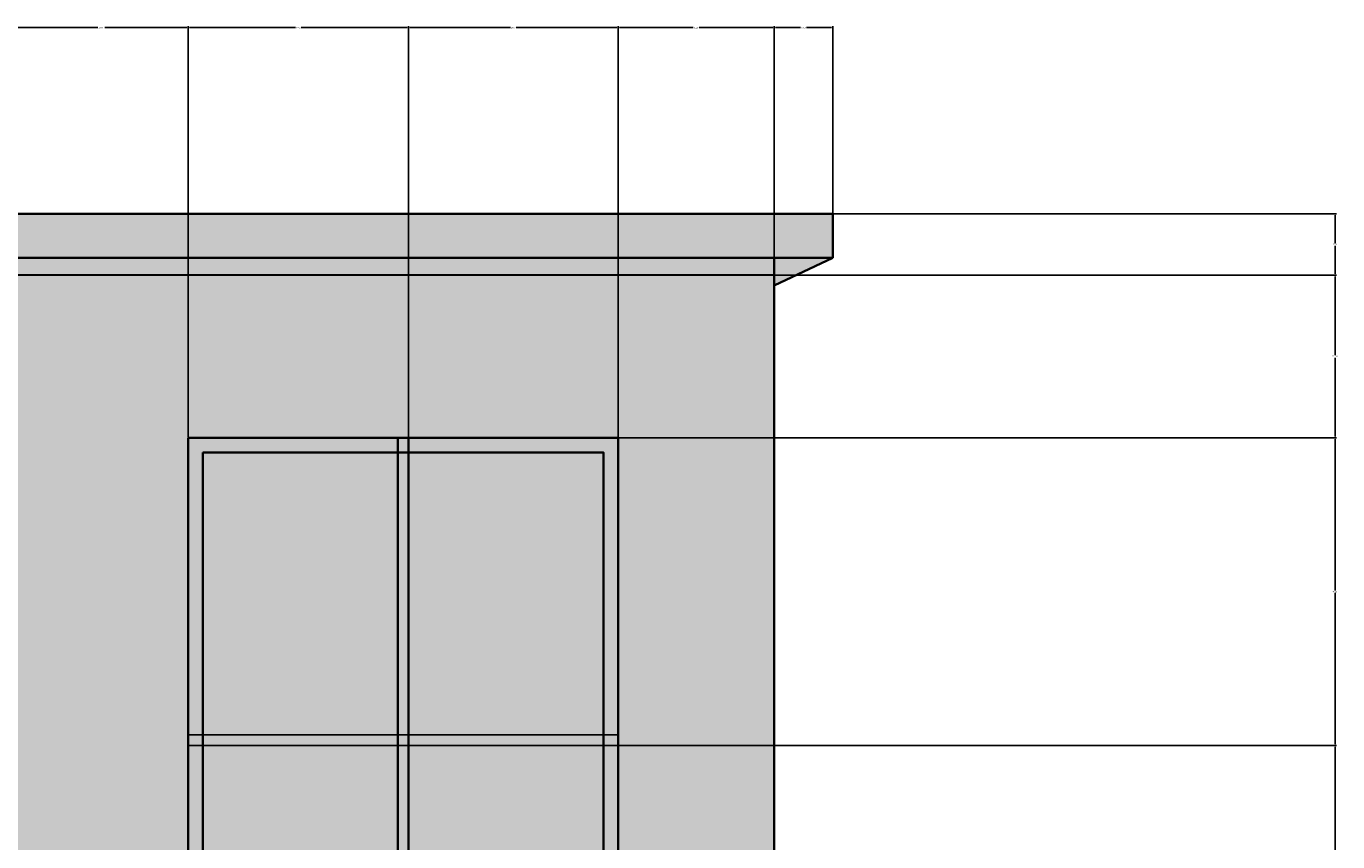
# Model space of a CAD drawing. Units: feet. Extents: x 2415 to 6174, y 866 to 1295.
# Tile 6 of 9: x 3580 to 3759, y 1184 to 1295. Entities that reach past the tile are written whole.
import ezdxf

# ---------------------------------------------------------------- set-up
doc = ezdxf.new("R2010")
doc.units = ezdxf.units.FT
for name, color, linetype, lineweight in [('A-ANNO-DIMS', 2, 'Continuous', 18), ('A-ELEV', 7, 'Continuous', 35), ('A-ELEV-PATT', 8, 'Continuous', 13), ('A-GLAZ', 4, 'Continuous', 25)]:
    doc.layers.add(name, color=color, linetype=linetype, lineweight=lineweight)
doc.styles.get("Standard").update_dxf_attribs({"font": 'arial.ttf'})
doc.dimstyles.get("Standard").update_dxf_attribs({"dimtxt": 0.18, "dimasz": 0.18, "dimexe": 0.18, "dimexo": 0.0625, "dimgap": 0.09, "dimtad": 0, "dimtih": 1, "dimtoh": 1, "dimdec": 1, "dimzin": 0, "dimdsep": 46, "dimlunit": 3, "dimtxsty": 'Standard', "dimcen": 0.09, "dimadec": 0, "dimazin": 0, "dimtfac": 1, "dimtdec": 1, "dimtofl": 0, "dimtmove": 0, "dimatfit": 3, "dimfxl": 1, "dimtolj": 1, "dimtzin": 0, "dimarcsym": 0})

# ---------------------------------------------------------------- blocks, each defined once
blk = doc.blocks.new('*D67')
at = {"layer": 'A-ANNO-DIMS', "color": 0, "lineweight": -2, "transparency": 16777216}
for p, q in [((3578.56, 1263.66), (3578.56, 1295.18)), ((3578.74, 1295), (3589.92, 1295)), ((3602.04, 1295), (3590.85, 1295)), ((3602.22, 1239.13), (3602.22, 1295.18))]:
    blk.add_line(p, q, dxfattribs=at)
at = {"layer": 'A-ANNO-DIMS', "color": 0, "transparency": 16777216}
for points in [[(3578.74, 1295.03), (3578.74, 1294.97), (3578.56, 1295)], [(3602.04, 1295.03), (3602.04, 1294.97), (3602.22, 1295)]]:
    blk.add_solid(points, dxfattribs=at)
at = {"layer": 'Defpoints', "color": 0, "transparency": 16777216}
for p in [(3602.22, 1295), (3578.56, 1263.6), (3602.22, 1239.07)]:
    blk.add_point(p, dxfattribs=at)
at = {"layer": 'A-ANNO-DIMS', "color": 0, "transparency": 16777216, "insert": (3590.39, 1295), "char_height": 0.18, "attachment_point": 5}
blk.add_mtext('\\A1;23.657', dxfattribs=at)
blk = doc.blocks.new('*D68')
at = {"layer": 'A-ANNO-DIMS', "color": 0, "lineweight": -2, "transparency": 16777216}
for p, q in [((3602.22, 1239.13), (3602.22, 1295.18)), ((3602.4, 1295), (3616.84, 1295)), ((3632.06, 1295), (3617.62, 1295)), ((3632.24, 1239.13), (3632.24, 1295.18))]:
    blk.add_line(p, q, dxfattribs=at)
at = {"layer": 'A-ANNO-DIMS', "color": 0, "transparency": 16777216}
for points in [[(3602.4, 1295.03), (3602.4, 1294.97), (3602.22, 1295)], [(3632.06, 1295.03), (3632.06, 1294.97), (3632.24, 1295)]]:
    blk.add_solid(points, dxfattribs=at)
at = {"layer": 'Defpoints', "color": 0, "transparency": 16777216}
for p in [(3632.24, 1295), (3602.22, 1239.07), (3632.24, 1239.07)]:
    blk.add_point(p, dxfattribs=at)
at = {"layer": 'A-ANNO-DIMS', "color": 0, "transparency": 16777216, "insert": (3617.23, 1295), "char_height": 0.18, "attachment_point": 5}
blk.add_mtext('\\A1;30.03', dxfattribs=at)
blk = doc.blocks.new('*D69')
at = {"layer": 'A-ANNO-DIMS', "color": 0, "lineweight": -2, "transparency": 16777216}
for p, q in [((3632.24, 1239.13), (3632.24, 1295.18)), ((3632.42, 1295), (3646.13, 1295)), ((3660.63, 1295), (3646.92, 1295)), ((3660.81, 1239.13), (3660.81, 1295.18))]:
    blk.add_line(p, q, dxfattribs=at)
at = {"layer": 'A-ANNO-DIMS', "color": 0, "transparency": 16777216}
for points in [[(3632.42, 1295.03), (3632.42, 1294.97), (3632.24, 1295)], [(3660.63, 1295.03), (3660.63, 1294.97), (3660.81, 1295)]]:
    blk.add_solid(points, dxfattribs=at)
at = {"layer": 'Defpoints', "color": 0, "transparency": 16777216}
for p in [(3660.81, 1295), (3632.24, 1239.07), (3660.81, 1239.07)]:
    blk.add_point(p, dxfattribs=at)
at = {"layer": 'A-ANNO-DIMS', "color": 0, "transparency": 16777216, "insert": (3646.53, 1295), "char_height": 0.18, "attachment_point": 5}
blk.add_mtext('\\A1;28.57', dxfattribs=at)
blk = doc.blocks.new('*D70')
at = {"layer": 'A-ANNO-DIMS', "color": 0, "lineweight": -2, "transparency": 16777216}
for p, q in [((3660.81, 1239.13), (3660.81, 1295.18)), ((3660.99, 1295), (3671.05, 1295)), ((3681.89, 1295), (3671.84, 1295)), ((3682.07, 1261.33), (3682.07, 1295.18))]:
    blk.add_line(p, q, dxfattribs=at)
at = {"layer": 'A-ANNO-DIMS', "color": 0, "transparency": 16777216}
for points in [[(3660.99, 1295.03), (3660.99, 1294.97), (3660.81, 1295)], [(3681.89, 1295.03), (3681.89, 1294.97), (3682.07, 1295)]]:
    blk.add_solid(points, dxfattribs=at)
at = {"layer": 'Defpoints', "color": 0, "transparency": 16777216}
for p in [(3682.07, 1295), (3682.07, 1261.26), (3660.81, 1239.07)]:
    blk.add_point(p, dxfattribs=at)
at = {"layer": 'A-ANNO-DIMS', "color": 0, "transparency": 16777216, "insert": (3671.44, 1295), "char_height": 0.18, "attachment_point": 5}
blk.add_mtext('\\A1;21.26', dxfattribs=at)
blk = doc.blocks.new('*D71')
at = {"layer": 'A-ANNO-DIMS', "color": 0, "lineweight": -2, "transparency": 16777216}
for p, q in [((3682.07, 1261.33), (3682.07, 1295.18)), ((3682.25, 1295), (3685.69, 1295)), ((3689.91, 1295), (3686.48, 1295)), ((3690.09, 1269.66), (3690.09, 1295.18))]:
    blk.add_line(p, q, dxfattribs=at)
at = {"layer": 'A-ANNO-DIMS', "color": 0, "transparency": 16777216}
for points in [[(3682.25, 1295.03), (3682.25, 1294.97), (3682.07, 1295)], [(3689.91, 1295.03), (3689.91, 1294.97), (3690.09, 1295)]]:
    blk.add_solid(points, dxfattribs=at)
at = {"layer": 'Defpoints', "color": 0, "transparency": 16777216}
for p in [(3690.09, 1295), (3690.09, 1269.6), (3682.07, 1261.26)]:
    blk.add_point(p, dxfattribs=at)
at = {"layer": 'A-ANNO-DIMS', "color": 0, "transparency": 16777216, "insert": (3686.08, 1295), "char_height": 0.18, "attachment_point": 5}
blk.add_mtext('\\A1;8.019', dxfattribs=at)
blk = doc.blocks.new('*D86')
at = {"layer": 'A-ANNO-DIMS', "color": 0, "lineweight": -2, "transparency": 16777216}
for p, q in [((3660.88, 1197.11), (3758.71, 1197.11)), ((3758.53, 1196.93), (3758.53, 1177.05)), ((3758.53, 1156.8), (3758.53, 1176.69)), ((3660.88, 1156.62), (3758.71, 1156.62))]:
    blk.add_line(p, q, dxfattribs=at)
at = {"layer": 'A-ANNO-DIMS', "color": 0, "transparency": 16777216}
for points in [[(3758.5, 1196.93), (3758.56, 1196.93), (3758.53, 1197.11)], [(3758.5, 1156.8), (3758.56, 1156.8), (3758.53, 1156.62)]]:
    blk.add_solid(points, dxfattribs=at)
at = {"layer": 'Defpoints', "color": 0, "transparency": 16777216}
for p in [(3660.81, 1197.11), (3758.53, 1197.11), (3660.81, 1156.62)]:
    blk.add_point(p, dxfattribs=at)
at = {"layer": 'A-ANNO-DIMS', "color": 0, "transparency": 16777216, "insert": (3758.53, 1176.87), "char_height": 0.18, "attachment_point": 5}
blk.add_mtext('\\A1;40.49', dxfattribs=at)
blk = doc.blocks.new('*D87')
at = {"layer": 'A-ANNO-DIMS', "color": 0, "lineweight": -2, "transparency": 16777216}
for p, q in [((3660.88, 1239.07), (3758.71, 1239.07)), ((3758.53, 1238.89), (3758.53, 1218.27)), ((3758.53, 1197.29), (3758.53, 1217.91)), ((3660.88, 1197.11), (3758.71, 1197.11))]:
    blk.add_line(p, q, dxfattribs=at)
at = {"layer": 'A-ANNO-DIMS', "color": 0, "transparency": 16777216}
for points in [[(3758.5, 1238.89), (3758.56, 1238.89), (3758.53, 1239.07)], [(3758.5, 1197.29), (3758.56, 1197.29), (3758.53, 1197.11)]]:
    blk.add_solid(points, dxfattribs=at)
at = {"layer": 'Defpoints', "color": 0, "transparency": 16777216}
for p in [(3660.81, 1239.07), (3758.53, 1239.07), (3660.81, 1197.11)]:
    blk.add_point(p, dxfattribs=at)
at = {"layer": 'A-ANNO-DIMS', "color": 0, "transparency": 16777216, "insert": (3758.53, 1218.09), "char_height": 0.18, "attachment_point": 5}
blk.add_mtext('\\A1;41.95', dxfattribs=at)
blk = doc.blocks.new('*D88')
at = {"layer": 'A-ANNO-DIMS', "color": 0, "lineweight": -2, "transparency": 16777216}
for p, q in [((3682.13, 1261.26), (3758.71, 1261.26)), ((3758.53, 1261.08), (3758.53, 1250.35)), ((3758.53, 1239.25), (3758.53, 1249.98)), ((3660.88, 1239.07), (3758.71, 1239.07))]:
    blk.add_line(p, q, dxfattribs=at)
at = {"layer": 'A-ANNO-DIMS', "color": 0, "transparency": 16777216}
for points in [[(3758.5, 1261.08), (3758.56, 1261.08), (3758.53, 1261.26)], [(3758.5, 1239.25), (3758.56, 1239.25), (3758.53, 1239.07)]]:
    blk.add_solid(points, dxfattribs=at)
at = {"layer": 'Defpoints', "color": 0, "transparency": 16777216}
for p in [(3682.07, 1261.26), (3758.53, 1261.26), (3660.81, 1239.07)]:
    blk.add_point(p, dxfattribs=at)
at = {"layer": 'A-ANNO-DIMS', "color": 0, "transparency": 16777216, "insert": (3758.53, 1250.16), "char_height": 0.18, "attachment_point": 5}
blk.add_mtext('\\A1;22.196', dxfattribs=at)
blk = doc.blocks.new('*D89')
at = {"layer": 'A-ANNO-DIMS', "color": 0, "lineweight": -2, "transparency": 16777216}
for p, q in [((3690.15, 1269.6), (3758.71, 1269.6)), ((3758.53, 1269.42), (3758.53, 1265.61)), ((3758.53, 1261.44), (3758.53, 1265.25)), ((3682.13, 1261.26), (3758.71, 1261.26))]:
    blk.add_line(p, q, dxfattribs=at)
at = {"layer": 'A-ANNO-DIMS', "color": 0, "transparency": 16777216}
for points in [[(3758.5, 1269.42), (3758.56, 1269.42), (3758.53, 1269.6)], [(3758.5, 1261.44), (3758.56, 1261.44), (3758.53, 1261.26)]]:
    blk.add_solid(points, dxfattribs=at)
at = {"layer": 'Defpoints', "color": 0, "transparency": 16777216}
for p in [(3690.09, 1269.6), (3758.53, 1269.6), (3682.07, 1261.26)]:
    blk.add_point(p, dxfattribs=at)
at = {"layer": 'A-ANNO-DIMS', "color": 0, "transparency": 16777216, "insert": (3758.53, 1265.43), "char_height": 0.18, "attachment_point": 5}
blk.add_mtext('\\A1;8.336', dxfattribs=at)

msp = doc.modelspace()

# ---------------------------------------------------------------- hatches: boundary and pattern name
at = {"layer": 'A-ELEV-PATT'}
h = msp.add_hatch(color=256, dxfattribs=at)
h.set_gradient(color1=(255, 255, 255), tint=1)
h.paths.add_polyline_path([(3264.916, 1143.5993), (3253.129, 1143.5993), (3253.129, 891.5993), (3264.916, 891.5993)])
h.paths.add_polyline_path([(3470.0448, 1143.5993), (3264.916, 1143.5993), (3264.916, 1137.5993), (3466.5999, 1137.5993)])
h.paths.add_polyline_path([(3363.8667, 1137.5993), (3264.916, 1137.5993), (3264.916, 1011.5993), (3363.8667, 1011.5993)])
h.paths.add_polyline_path([(3286.0429, 1117.0591), (3337.7904, 1117.0591), (3337.7904, 1115.4381), (3336.5314, 1115.4381), (3336.5314, 1110.528), (3335.4882, 1110.528), (3335.4882, 1042.3194), (3288.3452, 1042.3194), (3288.3452, 1110.528), (3287.3019, 1110.528), (3287.3019, 1115.4381), (3286.0429, 1115.4381)], flags=16)
h.paths.add_polyline_path([(3290.3452, 1108.528), (3333.4882, 1108.528), (3333.4882, 1044.3194), (3290.3452, 1044.3194)], flags=0)
h.paths.add_polyline_path([(3292.3452, 1106.528), (3331.4882, 1106.528), (3331.4882, 1046.3194), (3292.3452, 1046.3194)], flags=0)
h.paths.add_polyline_path([(3311.7156, 1106.528), (3312.1178, 1106.528), (3312.1178, 1046.3194), (3311.7156, 1046.3194)], flags=0)
h.paths.add_polyline_path([(3682.0722, 1263.5992), (3578.5579, 1263.5992), (3578.5579, 1137.5993), (3578.5579, 961.3655), (3682.0722, 961.3655)])
h.paths.add_polyline_path([(3660.8129, 1239.0671), (3660.8129, 996.6447), (3602.2151, 996.6447), (3602.2151, 1239.0671)], flags=16)
h.paths.add_polyline_path([(3632.2447, 1239.0671), (3632.2447, 996.6447), (3630.7833, 996.6447), (3630.7833, 1029.3019), (3602.2151, 1029.3019), (3602.2151, 1030.7632), (3630.7833, 1030.7632), (3630.7833, 1071.2549), (3602.2151, 1071.2549), (3602.2151, 1072.7163), (3630.7833, 1072.7163), (3630.7833, 1113.2079), (3602.2151, 1113.2079), (3602.2151, 1114.6693), (3630.7833, 1114.6693), (3630.7833, 1155.161), (3602.2151, 1155.161), (3602.2151, 1156.6224), (3630.7833, 1156.6224), (3630.7833, 1197.114), (3602.2151, 1197.114), (3602.2151, 1198.5754), (3630.7833, 1198.5754), (3630.7833, 1239.0671)], flags=0)
h.paths.add_polyline_path([(3733.129, 951.5993), (3634.5374, 951.5993), (3634.5374, 891.5993), (3733.129, 891.5993)])
h.paths.add_polyline_path([(3627.8799, 951.5993), (3621.0953, 951.5993), (3621.0953, 891.5993), (3627.8799, 891.5993)])
h.paths.add_polyline_path([(3614.4378, 951.5993), (3607.6532, 951.5993), (3607.6532, 891.5993), (3614.4378, 891.5993)])
h.paths.add_polyline_path([(3565.9347, 951.5993), (3441.3079, 951.5993), (3441.3079, 891.5993), (3565.9347, 891.5993)], flags=17)
h.paths.add_polyline_path([(3571.9347, 957.5993), (3435.3079, 957.5993), (3435.3079, 891.5993), (3441.3079, 891.5993), (3441.3079, 951.5993), (3565.9347, 951.5993), (3565.9347, 891.5993), (3571.9347, 891.5993)])
h.paths.add_polyline_path([(3435.3079, 1011.5993), (3423.5209, 1011.5993), (3423.5209, 891.5993), (3435.3079, 891.5993), (3435.3079, 957.5993)])
h.paths.add_polyline_path([(3690.0912, 1269.5992), (3571.9347, 1269.5992), (3571.9347, 1263.5992), (3690.0912, 1263.5992)])
h.paths.add_polyline_path([(3571.9347, 1269.5992), (3538.5122, 1257.6449), (3538.5122, 1251.6449), (3571.9347, 1263.5992)])
h = msp.add_hatch(color=256, dxfattribs=at)
h.set_gradient(color1=(205, 105, 40), color2=(205, 105, 40))
h.paths.add_polyline_path([(3682.0722, 1263.5992), (3578.5579, 1263.5992), (3578.5579, 1261.2323), (3682.0722, 1261.2628)])
h.paths.add_polyline_path([(3571.9347, 1261.2303), (3571.9347, 1263.5992), (3538.5122, 1251.6449), (3538.5466, 1251.5295), (3544.7493, 1251.5295), (3545.1353, 1251.6449)])
h.paths.add_polyline_path([(3578.5579, 1263.5992), (3571.9347, 1263.5992), (3571.9347, 1261.2303)])
h.paths.add_polyline_path([(3690.0912, 1263.5992), (3682.0722, 1263.5992), (3682.0722, 1261.2628), (3682.0722, 1259.8122)])
h = msp.add_hatch(color=256, dxfattribs=at)
h.set_gradient(color1=(99, 100, 102), color2=(99, 100, 102))
h.paths.add_polyline_path([(3660.8129, 1239.0671), (3602.2151, 1239.0671), (3602.2151, 996.6447), (3660.8129, 996.6447)])
h.paths.add_polyline_path([(3604.2151, 1237.0671), (3658.8129, 1237.0671), (3658.8129, 998.6447), (3604.2151, 998.6447)], flags=16)
h = msp.add_hatch(color=256, dxfattribs=at)
h.set_gradient(color1=(181, 210, 237), color2=(122, 175, 223))
h.paths.add_polyline_path([(3630.7833, 1239.0671), (3602.2151, 1239.0671), (3602.2151, 1198.5754), (3630.7833, 1198.5754)])
h.paths.add_polyline_path([(3660.8129, 1239.0671), (3632.2447, 1239.0671), (3632.2447, 1198.5754), (3660.8129, 1198.5754)])
h.paths.add_polyline_path([(3630.7833, 1197.114), (3602.2151, 1197.114), (3602.2151, 1156.6224), (3630.7833, 1156.6224)])
h.paths.add_polyline_path([(3660.8129, 1197.114), (3632.2447, 1197.114), (3632.2447, 1156.6224), (3660.8129, 1156.6224)])
h.paths.add_polyline_path([(3630.7833, 1155.161), (3602.2151, 1155.161), (3602.2151, 1114.6693), (3630.7833, 1114.6693)])
h.paths.add_polyline_path([(3660.8129, 1155.161), (3632.2447, 1155.161), (3632.2447, 1114.6693), (3660.8129, 1114.6693)])
h.paths.add_polyline_path([(3630.7833, 1113.2079), (3602.2151, 1113.2079), (3602.2151, 1072.7163), (3630.7833, 1072.7163)])
h.paths.add_polyline_path([(3660.8129, 1113.2079), (3632.2447, 1113.2079), (3632.2447, 1072.7163), (3660.8129, 1072.7163)])
h.paths.add_polyline_path([(3660.8129, 1071.2549), (3632.2447, 1071.2549), (3632.2447, 996.6447), (3660.8129, 996.6447)])
h.paths.add_polyline_path([(3630.7833, 1071.2549), (3602.2151, 1071.2549), (3602.2151, 1030.7632), (3630.7833, 1030.7632)])
h.paths.add_polyline_path([(3630.7833, 1029.3019), (3602.2151, 1029.3019), (3602.2151, 996.6447), (3630.7833, 996.6447)])
h = msp.add_hatch(color=256, dxfattribs=at)
h.set_gradient(color2=(0, 0, 0))
h.paths.add_polyline_path([(3630.7833, 1030.7632), (3604.2151, 1030.7632), (3604.2151, 1029.3019), (3630.7833, 1029.3019)])
h.paths.add_polyline_path([(3658.8129, 1030.7632), (3632.2447, 1030.7632), (3632.2447, 1029.3019), (3658.8129, 1029.3019)])
h.paths.add_polyline_path([(3632.2447, 1030.7632), (3630.7833, 1030.7632), (3630.7833, 1029.3019), (3632.2447, 1029.3019)])
h.paths.add_polyline_path([(3632.2447, 1239.0671), (3630.7833, 1239.0671), (3630.7833, 1030.7632), (3632.2447, 1030.7632)])
h.paths.add_polyline_path([(3632.2447, 1029.3019), (3630.7833, 1029.3019), (3630.7833, 996.6447), (3632.2447, 996.6447)])
h = msp.add_hatch(color=256, dxfattribs=at)
h.set_gradient(color2=(0, 0, 0))
h.paths.add_polyline_path([(3630.7833, 1198.5754), (3604.2151, 1198.5754), (3604.2151, 1197.114), (3630.7833, 1197.114)])
h.paths.add_polyline_path([(3658.8129, 1198.5754), (3632.2447, 1198.5754), (3632.2447, 1197.114), (3658.8129, 1197.114)])

# ---------------------------------------------------------------- linework, layer by layer
at = {"layer": 'A-ELEV'}
for p, q in [((3690.0912, 1269.5992), (3571.9347, 1269.5992)), ((3690.0912, 1269.5992), (3690.0912, 1263.5992)), ((3571.9347, 1263.5992), (3690.0912, 1263.5992)), ((3690.0912, 1263.5992), (3682.0722, 1259.8122)), ((3571.9347, 1261.2303), (3682.0722, 1261.2628))]:
    msp.add_line(p, q, dxfattribs=at)
msp.add_lwpolyline([(3682.0722, 1263.5992), (3682.0722, 961.3655), (3578.5579, 961.3655)], dxfattribs=at)
for points in [[(3602.2151, 1239.0671), (3660.8129, 1239.0671), (3660.8129, 996.6447), (3602.2151, 996.6447)], [(3630.7833, 1239.0671), (3632.2447, 1239.0671), (3632.2447, 996.6447), (3630.7833, 996.6447)], [(3604.2151, 1237.0671), (3658.8129, 1237.0671), (3658.8129, 998.6447), (3604.2151, 998.6447)]]:
    msp.add_lwpolyline(points, close=True, dxfattribs=at)
at = {"layer": 'A-GLAZ'}
msp.add_lwpolyline([(3660.8129, 1197.114), (3602.2151, 1197.114), (3602.2151, 1198.5754), (3660.8129, 1198.5754)], dxfattribs=at)

# ---------------------------------------------------------------- dimensions: what is measured, and where the dimension line sits
at = {"layer": 'A-ANNO-DIMS'}
for base, p1, p2, override, picture, middle in [((3602.2151, 1294.9993), (3578.5579, 1263.5992), (3602.2151, 1239.0671), {"dimdec": 3, "dimlfac": 1, "dimrnd": 0, "dimzin": 0, "dimdsep": 46, "dimlunit": 2}, '*D67', (3590.3865, 1294.9993)), ((3632.2447, 1294.9993), (3602.2151, 1239.0671), (3632.2447, 1239.0671), {"dimdec": 2, "dimlfac": 1, "dimrnd": 0, "dimzin": 0, "dimdsep": 46, "dimlunit": 2}, '*D68', (3617.2299, 1294.9993)), ((3660.8129, 1294.9993), (3632.2447, 1239.0671), (3660.8129, 1239.0671), {"dimdec": 2, "dimlfac": 1, "dimrnd": 0, "dimzin": 0, "dimdsep": 46, "dimlunit": 2}, '*D69', (3646.5288, 1294.9993)), ((3682.0722, 1294.9993), (3660.8129, 1239.0671), (3682.0722, 1261.2628), {"dimdec": 2, "dimlfac": 1, "dimrnd": 0, "dimzin": 0, "dimdsep": 46, "dimlunit": 2}, '*D70', (3671.4425, 1294.9993)), ((3690.0912, 1294.9993), (3682.0722, 1261.2628), (3690.0912, 1269.5992), {"dimdec": 3, "dimlfac": 1, "dimrnd": 0, "dimzin": 0, "dimdsep": 46, "dimlunit": 2}, '*D71', (3686.0817, 1294.9993))]:
    dim = msp.add_linear_dim(base=base, p1=p1, p2=p2, dimstyle='Standard', override=override, dxfattribs=at)
    dim.commit()
    dim.dimension.update_dxf_attribs({"geometry": picture, "text_midpoint": middle})
for base, p1, p2, override, picture, middle in [((3758.529, 1269.5992), (3682.0722, 1261.2628), (3690.0912, 1269.5992), {"dimdec": 3, "dimlfac": 1, "dimrnd": 0, "dimzin": 0, "dimdsep": 46, "dimlunit": 2}, '*D89', (3758.529, 1265.431)), ((3758.529, 1261.2628), (3660.8129, 1239.0671), (3682.0722, 1261.2628), {"dimdec": 3, "dimlfac": 1, "dimrnd": 0, "dimzin": 0, "dimdsep": 46, "dimlunit": 2}, '*D88', (3758.529, 1250.1649)), ((3758.529, 1239.0671), (3660.8129, 1197.114), (3660.8129, 1239.0671), {"dimdec": 2, "dimlfac": 1, "dimrnd": 0, "dimzin": 0, "dimdsep": 46, "dimlunit": 2}, '*D87', (3758.529, 1218.0905)), ((3758.529, 1197.114), (3660.8129, 1156.6224), (3660.8129, 1197.114), {"dimdec": 2, "dimlfac": 1, "dimrnd": 0, "dimzin": 0, "dimdsep": 46, "dimlunit": 2}, '*D86', (3758.529, 1176.8682))]:
    dim = msp.add_linear_dim(base=base, p1=p1, p2=p2, angle=90, dimstyle='Standard', override=override, dxfattribs=at)
    dim.commit()
    dim.dimension.update_dxf_attribs({"geometry": picture, "text_midpoint": middle})

doc.saveas('drawing.dxf')
